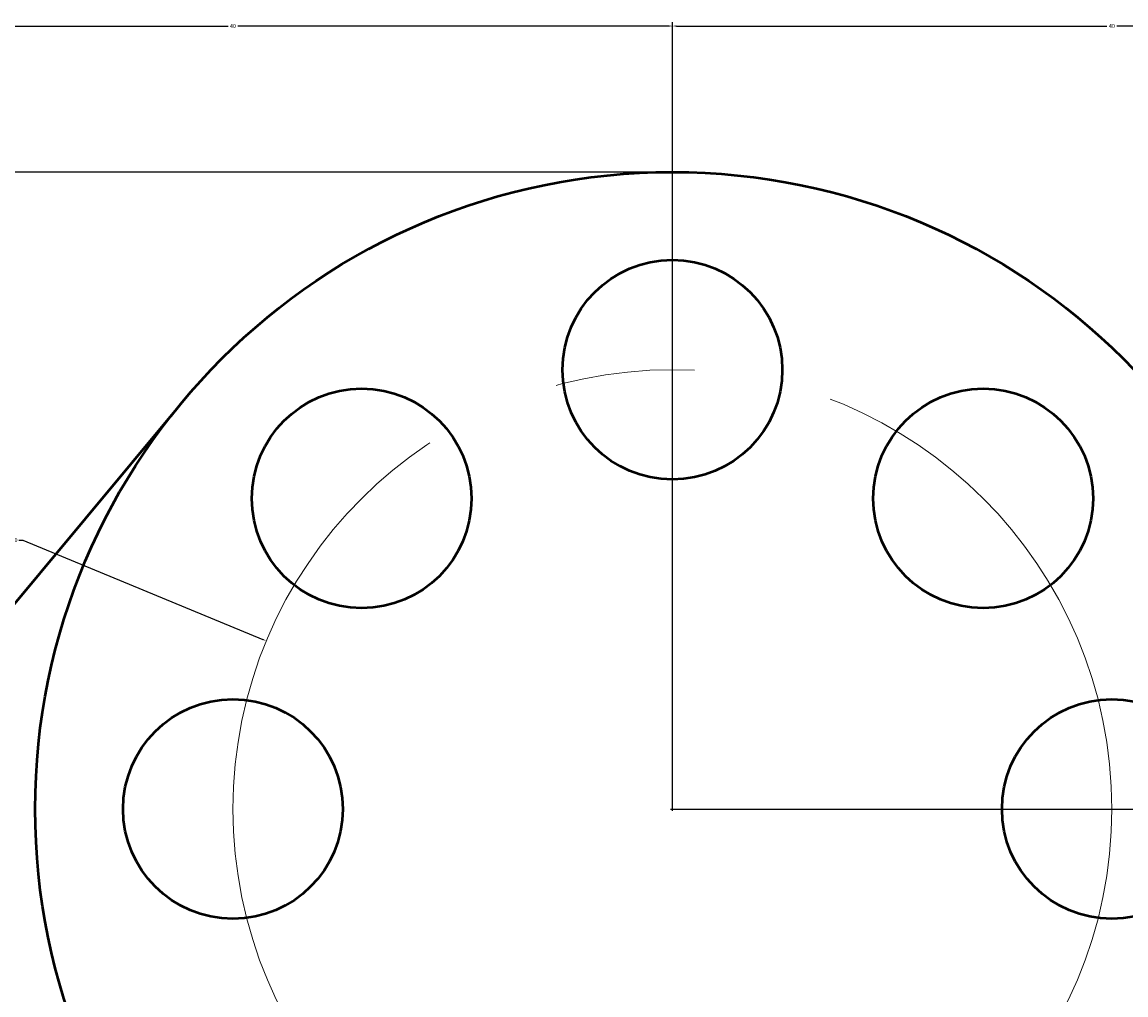
# Model space of a CAD drawing. Units: inches. Extents: x -11 to 126, y -62 to 82.
# Tile 9 of 10: x 30 to 80, y 38 to 82. Entities that reach past the tile are written whole.
import ezdxf

# ---------------------------------------------------------------- set-up
doc = ezdxf.new("R2010")
doc.units = ezdxf.units.IN
doc.header["$MEASUREMENT"] = 0
doc.linetypes.add('CENTER', pattern=[50.8, 31.75, -6.35, 6.35, -6.35])
for name, color, linetype, lineweight in [('M-CNTR', 4, 'CENTER', 18), ('M-DIMS', 2, 'Continuous', 18), ('M-OUTL', 7, 'Continuous', 50)]:
    doc.layers.add(name, color=color, linetype=linetype, lineweight=lineweight)
doc.styles.get("Standard").update_dxf_attribs({"font": 'arial.ttf'})
doc.dimstyles.get("Standard").update_dxf_attribs({"dimtxt": 0.18, "dimasz": 0.18, "dimexe": 0.18, "dimexo": 0.0625, "dimgap": 0.09, "dimtad": 0, "dimtih": 1, "dimtoh": 1, "dimdec": 4, "dimzin": 0, "dimdsep": 46, "dimtxsty": 'Standard', "dimcen": 0.09, "dimadec": 0, "dimazin": 0, "dimtfac": 1, "dimtdec": 4, "dimtofl": 0, "dimtmove": 0, "dimatfit": 3, "dimfxl": 1, "dimtolj": 1, "dimtzin": 0, "dimarcsym": 0})

# ---------------------------------------------------------------- blocks, each defined once
blk = doc.blocks.new('*U1')
blk.add_circle((0, 0), 5)
blk = doc.blocks.new('*U2')
at = {"layer": 'M-OUTL', "color": 0, "linetype": 'ByBlock', "lineweight": -2, "transparency": 16777216}
for p, rotation in [((59.232, 66.354), 180), ((45.089, 60.496), 225), ((73.374, 60.496), 135), ((39.232, 46.354), 270), ((79.232, 46.354), 90), ((45.089, 32.212), 315.0000000000001), ((73.374, 32.212), 44.99999999999998)]:
    blk.add_blockref('*U1', p, dxfattribs=dict(at, rotation=rotation))
blk.add_blockref('*U1', (59.232, 26.354), dxfattribs=at)
blk = doc.blocks.new('*D6')
at = {"layer": 'Defpoints', "color": 0, "transparency": 16777216}
for p in [(-7.399, 75.354), (59.232, 75.354), (59.232, -50.646)]:
    blk.add_point(p, dxfattribs=at)
at = {"layer": 'M-DIMS', "color": 0, "lineweight": -2, "transparency": 16777216}
for p, q in [((59.169, 75.354), (-7.579, 75.354)), ((-7.399, 75.174), (-7.399, 12.536)), ((-7.399, -50.466), (-7.399, 12.172)), ((59.169, -50.646), (-7.579, -50.646))]:
    blk.add_line(p, q, dxfattribs=at)
at = {"layer": 'M-DIMS', "color": 0, "transparency": 16777216}
for points in [[(-7.429, 75.174), (-7.369, 75.174), (-7.399, 75.354)], [(-7.429, -50.466), (-7.369, -50.466), (-7.399, -50.646)]]:
    blk.add_solid(points, dxfattribs=at)
at = {"layer": 'M-DIMS', "color": 0, "transparency": 16777216, "insert": (-7.399, 12.354), "char_height": 0.18, "attachment_point": 5}
blk.add_mtext('\\A1;126', dxfattribs=at)
blk = doc.blocks.new('*D7')
at = {"layer": 'Defpoints', "color": 0, "transparency": 16777216}
for p in [(59.232, 82.004), (59.232, 46.354), (19.232, 12.354)]:
    blk.add_point(p, dxfattribs=at)
at = {"layer": 'M-DIMS', "color": 0, "lineweight": -2, "transparency": 16777216}
for p, q in [((19.232, 12.417), (19.232, 82.184)), ((19.412, 82.004), (39.009, 82.004)), ((59.052, 82.004), (39.454, 82.004)), ((59.232, 46.417), (59.232, 82.184))]:
    blk.add_line(p, q, dxfattribs=at)
at = {"layer": 'M-DIMS', "color": 0, "transparency": 16777216}
for points in [[(19.412, 82.034), (19.412, 81.974), (19.232, 82.004)], [(59.052, 82.034), (59.052, 81.974), (59.232, 82.004)]]:
    blk.add_solid(points, dxfattribs=at)
at = {"layer": 'M-DIMS', "color": 0, "transparency": 16777216, "insert": (39.232, 82.004), "char_height": 0.18, "attachment_point": 5}
blk.add_mtext('\\A1;40', dxfattribs=at)
blk = doc.blocks.new('*D8')
at = {"layer": 'Defpoints', "color": 0, "transparency": 16777216}
for p in [(99.232, 82.004), (59.232, 46.354), (99.232, 12.354)]:
    blk.add_point(p, dxfattribs=at)
at = {"layer": 'M-DIMS', "color": 0, "lineweight": -2, "transparency": 16777216}
for p, q in [((59.232, 46.417), (59.232, 82.184)), ((59.412, 82.004), (79.009, 82.004)), ((99.052, 82.004), (79.454, 82.004)), ((99.232, 12.417), (99.232, 82.184))]:
    blk.add_line(p, q, dxfattribs=at)
at = {"layer": 'M-DIMS', "color": 0, "transparency": 16777216}
for points in [[(59.412, 82.034), (59.412, 81.974), (59.232, 82.004)], [(99.052, 82.034), (99.052, 81.974), (99.232, 82.004)]]:
    blk.add_solid(points, dxfattribs=at)
at = {"layer": 'M-DIMS', "color": 0, "transparency": 16777216, "insert": (79.232, 82.004), "char_height": 0.18, "attachment_point": 5}
blk.add_mtext('\\A1;40', dxfattribs=at)
blk = doc.blocks.new('*D10')
at = {"layer": 'Defpoints', "color": 0, "transparency": 16777216}
for p in [(59.232, 46.354), (125.882, 46.354), (99.232, 12.354)]:
    blk.add_point(p, dxfattribs=at)
at = {"layer": 'M-DIMS', "color": 0, "lineweight": -2, "transparency": 16777216}
for p, q in [((59.294, 46.354), (126.062, 46.354)), ((125.882, 46.174), (125.882, 29.536)), ((125.882, 12.534), (125.882, 29.172)), ((99.294, 12.354), (126.062, 12.354))]:
    blk.add_line(p, q, dxfattribs=at)
at = {"layer": 'M-DIMS', "color": 0, "transparency": 16777216}
for points in [[(125.852, 46.174), (125.912, 46.174), (125.882, 46.354)], [(125.852, 12.534), (125.912, 12.534), (125.882, 12.354)]]:
    blk.add_solid(points, dxfattribs=at)
at = {"layer": 'M-DIMS', "color": 0, "transparency": 16777216, "insert": (125.882, 29.354), "char_height": 0.18, "attachment_point": 5}
blk.add_mtext('\\A1;34', dxfattribs=at)
blk = doc.blocks.new('*D14')
at = {"layer": 'Defpoints', "color": 0, "transparency": 16777216}
for p in [(40.754, 54.008), (77.709, 38.701)]:
    blk.add_point(p, dxfattribs=at)
at = {"layer": 'M-DIMS', "color": 0, "lineweight": -2, "transparency": 16777216}
for p, q in [((29.487, 58.6), (29.667, 58.6)), ((29.667, 58.6), (40.588, 54.077)), ((59.142, 46.354), (59.322, 46.354)), ((59.232, 46.264), (59.232, 46.444))]:
    blk.add_line(p, q, dxfattribs=at)
at = {"layer": 'M-DIMS', "color": 0, "transparency": 16777216}
blk.add_solid([(40.599, 54.105), (40.576, 54.049), (40.754, 54.008)], dxfattribs=at)
at = {"layer": 'M-DIMS', "color": 0, "transparency": 16777216, "insert": (29.171, 58.6), "char_height": 0.18, "attachment_point": 5}
blk.add_mtext('\\A1;∅40', dxfattribs=at)

msp = doc.modelspace()

# ---------------------------------------------------------------- linework, layer by layer
at = {"layer": 'M-CNTR'}
msp.add_circle((59.232, 46.354), 20, dxfattribs=at)
at = {"layer": 'M-OUTL'}
msp.add_line((3.94, 25.244), (36.676, 64.582), dxfattribs=at)
msp.add_circle((59.232, 46.354), 29, dxfattribs=at)

# ---------------------------------------------------------------- block references
msp.add_blockref('*U2', (0, 0), dxfattribs=at)

# ---------------------------------------------------------------- dimensions: what is measured, and where the dimension line sits
at = {"layer": 'M-DIMS'}
for base, p1, p2, picture, middle in [((59.232, 82.004), (19.232, 12.354), (59.232, 46.354), '*D7', (39.232, 82.004)), ((99.232, 82.004), (59.232, 46.354), (99.232, 12.354), '*D8', (79.232, 82.004))]:
    dim = msp.add_linear_dim(base=base, p1=p1, p2=p2, dimstyle='Standard', override={"dimdec": 0, "dimlfac": 1, "dimrnd": 0, "dimzin": 0, "dimdsep": 46, "dimlunit": 2}, dxfattribs=at)
    dim.commit()
    dim.dimension.update_dxf_attribs({"geometry": picture, "text_midpoint": middle})
for base, p1, p2, picture, middle in [((-7.399, 75.354), (59.232, -50.646), (59.232, 75.354), '*D6', (-7.399, 12.354)), ((125.882, 46.354), (99.232, 12.354), (59.232, 46.354), '*D10', (125.882, 29.354))]:
    dim = msp.add_linear_dim(base=base, p1=p1, p2=p2, angle=90, dimstyle='Standard', override={"dimdec": 0, "dimlfac": 1, "dimrnd": 0, "dimzin": 0, "dimdsep": 46, "dimlunit": 2}, dxfattribs=at)
    dim.commit()
    dim.dimension.update_dxf_attribs({"geometry": picture, "text_midpoint": middle})
dim = msp.add_diameter_dim_2p(p1=(77.709, 38.701), p2=(40.754, 54.008), dimstyle='Standard', override={"dimdec": 0, "dimlfac": 1, "dimrnd": 0, "dimzin": 0, "dimdsep": 46, "dimlunit": 2}, dxfattribs=at)
dim.commit()
dim.dimension.update_dxf_attribs({"geometry": '*D14', "text_midpoint": (29.171, 58.6), "dimtype": 163})

doc.saveas('drawing.dxf')
